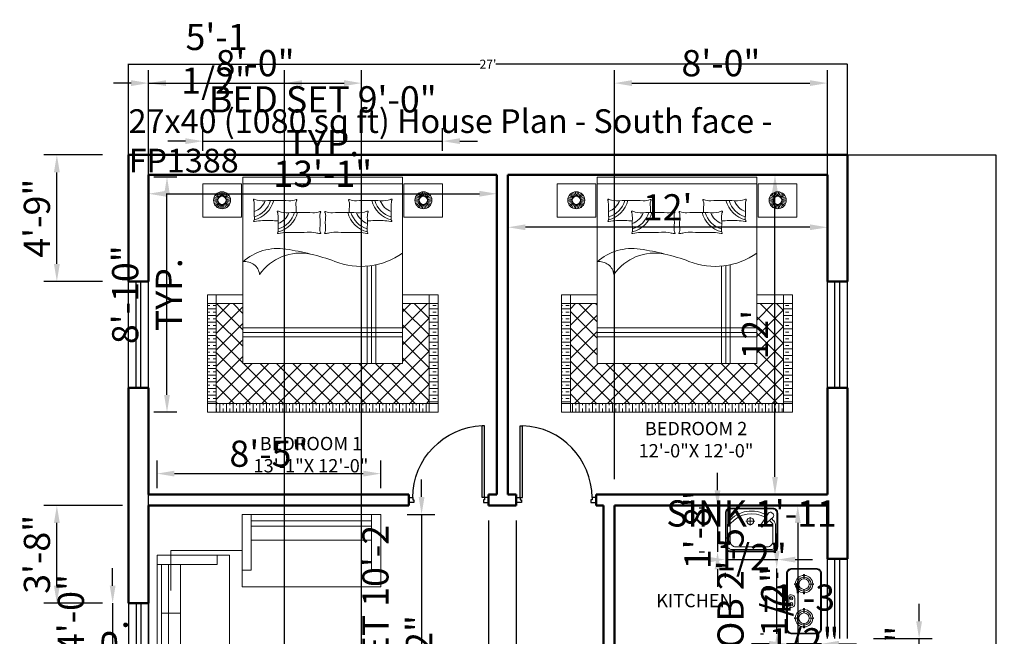
# Model space of a CAD drawing. Units: inches. Extents: x 117606 to 118050, y 251709 to 252357.
# Tile 3 of 3: x 117606 to 118050, y 252079 to 252357. Entities that reach past the tile are written whole.
import ezdxf

# ---------------------------------------------------------------- set-up
doc = ezdxf.new("R2010")
doc.units = ezdxf.units.IN
doc.header["$MEASUREMENT"] = 0
for name, color, linetype, lineweight in [('A-ANNO-TEXT', 7, 'Continuous', 25), ('A-AREA-IDEN', 7, 'Continuous', 25), ('A-DOOR', 4, 'Continuous', 25), ('A-EQPM', 9, 'Continuous', 18), ('FURNITURE', 53, 'Continuous', 18), ('SANITARY', 151, 'Continuous', 18), ('WALL', 7, 'Continuous', 50), ('WINDOW', 2, 'Continuous', 25), ('YQ_DIM', 3, 'Continuous', 18)]:
    doc.layers.add(name, color=color, linetype=linetype, lineweight=lineweight)
doc.styles.get("Standard").update_dxf_attribs({"font": 'arial.ttf'})
doc.styles.add('YQ_DIM', font='SUPEROS.SHX', dxfattribs={"width": 0.8, "bigfont": 'HZDX.SHX'})
doc.dimstyles.get("Standard").update_dxf_attribs({"dimtxt": 4, "dimasz": 0.18, "dimexe": 0.18, "dimexo": 0.0625, "dimgap": 0.09, "dimtad": 0, "dimtih": 1, "dimtoh": 1, "dimzin": 0, "dimdsep": 46, "dimlunit": 4, "dimtxsty": 'Standard', "dimcen": 0.09, "dimadec": 0, "dimazin": 0, "dimtfac": 1, "dimtofl": 0, "dimtmove": 0, "dimatfit": 3, "dimfxl": 1, "dimtolj": 1, "dimtzin": 0, "dimarcsym": 0})
doc.dimstyles.new('yqi3_937', dxfattribs={"dimscale": 3.937008, "dimtxt": 3, "dimasz": 2, "dimexe": 1.5, "dimexo": 3, "dimgap": 0.5, "dimtad": 1, "dimdsep": 46, "dimlunit": 4, "dimtxsty": 'YQ_DIM', "dimcen": 0, "dimclrd": 256, "dimclre": 256, "dimclrt": 7, "dimadec": 1, "dimazin": 2, "dimtfac": 1, "dimtix": 1, "dimtmove": 2, "dimatfit": 2, "dimfxl": 1, "dimtolj": 1, "dimtzin": 0, "dimarcsym": 0})

# ---------------------------------------------------------------- blocks, each defined once
blk = doc.blocks.new('*D1')
at = {"layer": 'Defpoints', "color": 0, "transparency": 16777216}
for p in [(117978.89, 252337.19), (117654.89, 252296.28), (117978.89, 252296.28)]:
    blk.add_point(p, dxfattribs=at)
at = {"layer": 'YQ_DIM', "color": 0, "lineweight": -2, "transparency": 16777216}
for p, q in [((117654.89, 252296.35), (117654.89, 252337.37)), ((117655.07, 252337.19), (117813.37, 252337.19)), ((117978.71, 252337.19), (117820.4, 252337.19)), ((117978.89, 252296.35), (117978.89, 252337.37))]:
    blk.add_line(p, q, dxfattribs=at)
at = {"layer": 'YQ_DIM', "color": 0, "transparency": 16777216}
for points in [[(117655.07, 252337.22), (117655.07, 252337.16), (117654.89, 252337.19)], [(117978.71, 252337.22), (117978.71, 252337.16), (117978.89, 252337.19)]]:
    blk.add_solid(points, dxfattribs=at)
at = {"layer": 'YQ_DIM', "color": 0, "transparency": 16777216, "insert": (117816.89, 252337.19), "char_height": 4, "attachment_point": 5}
blk.add_mtext("\\A1;27'", dxfattribs=at)
blk = doc.blocks.new('*D2')
at = {"layer": 'Defpoints', "color": 0, "transparency": 16777216}
for p in [(117978.89, 252296.28), (117978.89, 251816.28), (118045.85, 251816.28)]:
    blk.add_point(p, dxfattribs=at)
at = {"layer": 'YQ_DIM', "color": 0, "lineweight": -2, "transparency": 16777216}
for p, q in [((117978.95, 252296.28), (118046.03, 252296.28)), ((118045.85, 252296.1), (118045.85, 252058.42)), ((118045.85, 251816.46), (118045.85, 252054.15)), ((117978.95, 251816.28), (118046.03, 251816.28))]:
    blk.add_line(p, q, dxfattribs=at)
at = {"layer": 'YQ_DIM', "color": 0, "transparency": 16777216}
for points in [[(118045.82, 252296.1), (118045.88, 252296.1), (118045.85, 252296.28)], [(118045.82, 251816.46), (118045.88, 251816.46), (118045.85, 251816.28)]]:
    blk.add_solid(points, dxfattribs=at)
at = {"layer": 'YQ_DIM', "color": 0, "transparency": 16777216, "insert": (118045.85, 252056.28), "char_height": 4, "attachment_point": 5}
blk.add_mtext("\\A1;40'", dxfattribs=at)
blk = doc.blocks.new('*D4')
at = {"layer": 'Defpoints', "color": 0, "transparency": 16777216}
for p in [(117825.89, 252287.28), (117969.89, 252287.28), (117825.89, 252263.66)]:
    blk.add_point(p, dxfattribs=at)
at = {"layer": 'YQ_DIM', "color": 0, "lineweight": -2, "transparency": 16777216}
for p, q in [((117825.89, 252275.47), (117825.89, 252257.76)), ((117969.89, 252275.47), (117969.89, 252257.76)), ((117962.01, 252263.66), (117833.76, 252263.66))]:
    blk.add_line(p, q, dxfattribs=at)
at = {"layer": 'YQ_DIM', "color": 0, "transparency": 16777216}
for points in [[(117833.76, 252264.97), (117833.76, 252262.35), (117825.89, 252263.66)], [(117962.01, 252264.97), (117962.01, 252262.35), (117969.89, 252263.66)]]:
    blk.add_solid(points, dxfattribs=at)
at = {"layer": 'YQ_DIM', "color": 0, "transparency": 16777216, "insert": (117897.89, 252272.66), "char_height": 11.811, "attachment_point": 5, "style": 'YQ_DIM'}
blk.add_mtext("\\A1;12'", dxfattribs=at)
blk = doc.blocks.new('*D5')
at = {"layer": 'Defpoints', "color": 0, "transparency": 16777216}
for p in [(117946.26, 252287.28), (117969.89, 252287.28), (117969.89, 252143.28)]:
    blk.add_point(p, dxfattribs=at)
at = {"layer": 'YQ_DIM', "color": 0, "lineweight": -2, "transparency": 16777216}
for p, q in [((117958.07, 252287.28), (117940.36, 252287.28)), ((117946.26, 252151.16), (117946.26, 252279.41)), ((117958.07, 252143.28), (117940.36, 252143.28))]:
    blk.add_line(p, q, dxfattribs=at)
at = {"layer": 'YQ_DIM', "color": 0, "transparency": 16777216}
for points in [[(117944.95, 252279.41), (117947.58, 252279.41), (117946.26, 252287.28)], [(117944.95, 252151.16), (117947.58, 252151.16), (117946.26, 252143.28)]]:
    blk.add_solid(points, dxfattribs=at)
at = {"layer": 'YQ_DIM', "color": 0, "transparency": 16777216, "insert": (117937.26, 252215.28), "char_height": 11.811, "attachment_point": 5, "rotation": 90, "style": 'YQ_DIM'}
blk.add_mtext("\\A1;12'", dxfattribs=at)
blk = doc.blocks.new('*D9')
at = {"layer": 'Defpoints', "color": 0, "transparency": 16777216}
for p in [(117969.89, 252138.28), (117956.53, 252054.28), (117969.89, 252054.28)]:
    blk.add_point(p, dxfattribs=at)
at = {"layer": 'YQ_DIM', "color": 0, "lineweight": -2, "transparency": 16777216}
for p, q in [((117958.07, 252138.28), (117950.63, 252138.28)), ((117956.53, 252130.41), (117956.53, 252062.16)), ((117958.07, 252054.28), (117950.63, 252054.28))]:
    blk.add_line(p, q, dxfattribs=at)
at = {"layer": 'YQ_DIM', "color": 0, "transparency": 16777216}
for points in [[(117955.22, 252130.41), (117957.84, 252130.41), (117956.53, 252138.28)], [(117955.22, 252062.16), (117957.84, 252062.16), (117956.53, 252054.28)]]:
    blk.add_solid(points, dxfattribs=at)
at = {"layer": 'YQ_DIM', "color": 0, "transparency": 16777216, "insert": (117947.53, 252096.28), "char_height": 11.811, "attachment_point": 5, "rotation": 90, "style": 'YQ_DIM'}
blk.add_mtext("\\A1;7'", dxfattribs=at)
blk = doc.blocks.new('DR_D01')
for p, q in [((-0.45, 0.93), (-0.42, 0.93)), ((-0.45, 0.03), (-0.45, 0.93)), ((-0.42, 0.03), (-0.42, 0.93)), ((-0.5, 0.03), (-0.42, 0.03)), ((-0.5, 0.03), (-0.5, -0.03)), ((-0.45, 0.03), (-0.45, 0)), ((-0.45, 0), (-0.435, 0)), ((-0.435, 0), (-0.435, -0.03)), ((0.435, 0), (0.435, -0.03)), ((0.45, 0), (0.435, 0)), ((0.45, 0.03), (0.45, 0)), ((0.5, 0.03), (0.45, 0.03)), ((0.5, -0.03), (0.5, 0.03)), ((-0.435, -0.03), (-0.5, -0.03)), ((0.435, -0.03), (0.5, -0.03))]:
    blk.add_line(p, q)
blk.add_arc((-0.46, 0.021), 0.91, 0.5915, 87.4664)
blk = doc.blocks.new('WD_WIN4')
for p, q in [((-0.5, 0.5), (0.5, 0.5)), ((-0.5, 0.12), (0.5, 0.12)), ((-0.5, -0.12), (0.5, -0.12)), ((-0.5, -0.5), (0.5, -0.5))]:
    blk.add_line(p, q)
blk = doc.blocks.new('BED')
h = blk.add_hatch()
h.set_pattern_fill('TRANS', color=256, scale=12, style=0)
h.set_pattern_definition([(360, (4433.967, -9715.0492), (1e-15, 3), []), (360, (4433.967, -9713.5492), (1e-15, 3), [1.5, -1.5])])
h.paths.add_polyline_path([(48, -103), (52, -103), (52, -58), (48, -58)])
h.paths.add_polyline_path([(-48, -58), (-52, -58), (-52, -103), (-48, -103)])
h = blk.add_hatch()
h.set_pattern_fill('ANSI37', color=256, scale=42, angle=-90, style=0)
h.set_pattern_definition([(315, (7787.1367, 4477.8466), (3.7123106, 3.7123106), []), (45, (7787.1367, 4477.8466), (-3.7123106, 3.7123106), [])])
h.paths.add_polyline_path([(-36, -85), (-36, -58), (-48, -58), (-48, -103), (48, -103), (48, -58), (36, -58), (36, -85)])
h = blk.add_hatch()
h.set_pattern_fill('TRANS', color=256, scale=12, angle=-90, style=0)
h.set_pattern_definition([(270, (4433.967, -9715.0492), (3, -1e-15), []), (270, (4435.467, -9715.0492), (3, -1e-15), [1.5, -1.5])])
h.paths.add_polyline_path([(48, -107), (48, -103), (-48, -103), (-48, -107)])
for p, q in [((-54, -4), (-54, -19)), ((-36.64, -4), (-54, -4)), ((-36.64, -4), (-36.64, -19)), ((-36, -1), (36, -1)), ((-36, -85), (-36, -1)), ((-36, -4), (36, -4)), ((36, -1), (36, -85)), ((36.64, -4), (36.64, -19)), ((36.64, -4), (54, -4)), ((54, -4), (54, -19)), ((-46.62, -10.08), (-47.96, -8.6)), ((-46.31, -9.86), (-47.31, -8.13)), ((-45.96, -9.7), (-46.58, -7.8)), ((-45.58, -9.62), (-45.8, -7.63)), ((-45.2, -9.62), (-45, -7.63)), ((-44.82, -9.7), (-44.21, -7.79)), ((-44.47, -9.85), (-43.48, -8.12)), ((-44.16, -10.08), (-42.83, -8.59)), ((44.16, -10.08), (42.83, -8.59)), ((44.47, -9.85), (43.48, -8.12)), ((44.82, -9.7), (44.21, -7.79)), ((45.2, -9.62), (45, -7.63)), ((45.58, -9.62), (45.8, -7.63)), ((45.96, -9.7), (46.58, -7.8)), ((46.31, -9.86), (47.31, -8.13)), ((46.62, -10.08), (47.96, -8.6)), ((-47.23, -11.45), (-49.23, -11.45)), ((-47.19, -11.07), (-49.14, -10.66)), ((-47.19, -11.83), (-49.14, -12.25)), ((-47.07, -10.7), (-48.9, -9.89)), ((-47.07, -12.2), (-48.89, -13.01)), ((-46.88, -10.37), (-48.5, -9.2)), ((-46.87, -12.53), (-48.49, -13.71)), ((-46.62, -12.81), (-47.95, -14.3)), ((-46.3, -13.04), (-47.3, -14.77)), ((-45.95, -13.2), (-46.57, -15.1)), ((-45.58, -13.27), (-45.78, -15.26)), ((-45.19, -13.27), (-44.98, -15.26)), ((-44.82, -13.19), (-44.2, -15.09)), ((-44.47, -13.04), (-43.46, -14.77)), ((-44.16, -12.81), (-42.82, -14.29)), ((-43.9, -10.36), (-42.29, -9.18)), ((-43.9, -12.52), (-42.28, -13.7)), ((-43.71, -10.7), (-41.89, -9.88)), ((-43.71, -12.19), (-41.88, -13)), ((-43.59, -11.06), (-41.64, -10.64)), ((-43.59, -11.83), (-41.63, -12.24)), ((-43.55, -11.44), (-41.55, -11.44)), ((43.55, -11.44), (41.55, -11.44)), ((43.59, -11.83), (41.63, -12.24)), ((43.59, -11.06), (41.64, -10.64)), ((43.71, -12.19), (41.88, -13)), ((43.71, -10.7), (41.89, -9.88)), ((43.9, -12.52), (42.28, -13.7)), ((43.9, -10.36), (42.29, -9.18)), ((44.16, -12.81), (42.82, -14.29)), ((44.47, -13.04), (43.46, -14.77)), ((44.82, -13.19), (44.2, -15.09)), ((45.19, -13.27), (44.98, -15.26)), ((45.58, -13.27), (45.78, -15.26)), ((45.95, -13.2), (46.57, -15.1)), ((46.3, -13.04), (47.3, -14.77)), ((46.62, -12.81), (47.95, -14.3)), ((46.87, -12.53), (48.49, -13.71)), ((46.88, -10.37), (48.5, -9.2)), ((47.07, -10.7), (48.9, -9.89)), ((47.07, -12.2), (48.89, -13.01)), ((47.19, -11.07), (49.14, -10.66)), ((47.19, -11.83), (49.14, -12.25)), ((47.23, -11.45), (49.23, -11.45)), ((-36.64, -19), (-54, -19)), ((36.64, -19), (54, -19)), ((20, -85), (20, -41.14)), ((22, -85), (22, -40.91)), ((24, -85), (24, -40.55)), ((-52, -54), (-52, -107)), ((-52, -54), (-36, -54)), ((-48, -54), (-48, -107)), ((36, -54), (52, -54)), ((48, -54), (48, -107)), ((52, -54), (52, -107)), ((-52, -58), (-36, -58)), ((36, -58), (52, -58)), ((36, -69), (-36, -69)), ((36, -71), (-36, -71)), ((36, -73), (-36, -73)), ((36, -85), (-36, -85)), ((-52, -103), (52, -103)), ((-52, -107), (52, -107))]:
    blk.add_line(p, q)
for centre, radius in [((-45.39, -11.45), 3.84), ((45.39, -11.45), 3.84), ((-45.39, -11.45), 1.84), ((45.39, -11.45), 1.84)]:
    blk.add_circle(centre, radius)
for centre, radius, start, end in [((-30.92, -11.24), 0.328, 35.8976, 208.6272), ((-42.38, -17.5), 12.73, 27.1629, 28.6272), ((-44.37, -13.89), 13.5, 357.4804, 9.3956), ((-33.8, -8.61), 8.46, 289.8695, 338.9843), ((-33.8, -8.61), 12.06, 283.8498, 346.0842), ((-33.8, -8.61), 10.71, 286.0319, 344.1205), ((-26.84, 0.13), 11.82, 251.1782, 273.3982), ((-20.92, -99.64), 88.13, 86.2964, 93.3982), ((-14.79, -4.98), 6.73, 266.2964, 294.303), ((-8.24, -13.16), 3.86, 159.0146, 186.273), ((-11.92, -11.33), 0.242, 335.7259, 114.303), ((-5.69, -14.14), 6.59, 155.7259, 159.0146), ((11.92, -11.33), 0.242, 65.697, 204.2741), ((5.69, -14.14), 6.59, 20.9854, 24.2741), ((8.24, -13.16), 3.86, 353.727, 20.9854), ((14.79, -4.98), 6.73, 245.697, 273.7036), ((20.92, -99.64), 88.13, 86.6018, 93.7036), ((33.8, -8.61), 12.06, 193.9158, 256.1502), ((33.8, -8.61), 10.71, 195.8795, 253.9681), ((33.8, -8.61), 8.46, 201.0157, 250.1305), ((26.84, 0.13), 11.82, 266.6018, 288.8218), ((30.92, -11.24), 0.328, 331.3728, 144.1024), ((44.37, -13.89), 13.5, 170.6044, 182.5196), ((42.38, -17.5), 12.73, 151.3728, 152.8371), ((10.15, -16.29), 41.07, 177.4804, 184.5075), ((-20.16, -16.62), 0.328, 35.8976, 208.6272), ((-31.62, -22.87), 12.73, 27.1629, 28.6272), ((-33.61, -19.26), 13.5, 357.4804, 9.3956), ((-23.04, -13.99), 8.46, 289.8695, 338.9843), ((-23.04, -13.99), 12.06, 283.8498, 346.0842), ((-23.04, -13.99), 10.71, 286.0319, 344.1205), ((-16.08, -5.24), 11.82, 251.1782, 273.3982), ((-10.15, -105.01), 88.13, 86.2964, 93.3982), ((-36.64, -16.28), 24.71, 358.5721, 6.273), ((-4.03, -10.35), 6.73, 266.2964, 294.303), ((2.52, -18.53), 3.86, 159.0146, 186.273), ((-1.16, -16.7), 0.242, 335.7259, 114.303), ((5.07, -19.51), 6.59, 155.7259, 159.0146), ((1.16, -16.7), 0.242, 65.697, 204.2741), ((-5.07, -19.51), 6.59, 20.9854, 24.2741), ((-2.52, -18.53), 3.86, 353.727, 20.9854), ((4.03, -10.35), 6.73, 245.697, 273.7036), ((10.15, -105.01), 88.13, 86.6018, 93.7036), ((23.04, -13.99), 12.06, 193.9158, 256.1502), ((36.64, -16.28), 24.71, 173.727, 181.4279), ((23.04, -13.99), 10.71, 195.8795, 253.9681), ((23.04, -13.99), 8.46, 201.0157, 250.1305), ((16.08, -5.24), 11.82, 266.6018, 288.8218), ((20.16, -16.62), 0.328, 331.3728, 144.1024), ((33.61, -19.26), 13.5, 170.6044, 182.5196), ((31.62, -22.87), 12.73, 151.3728, 152.8371), ((-10.15, -16.29), 41.07, 355.4925, 2.5196), ((-30.88, -20.82), 0.25, 147.6219, 311.9343), ((-32.72, -19.65), 1.93, 327.6219, 339.2246), ((-32.67, -19.67), 1.88, 339.2246, 4.5075), ((-25.16, -53.53), 33, 93.5164, 99.6766), ((-25.27, -51.86), 31.33, 86.4836, 93.5164), ((-21.12, 15.68), 36.34, 266.4836, 271.5234), ((20.91, -21.66), 41.07, 177.4804, 184.5075), ((-25.88, -21.66), 24.71, 354.3784, 6.273), ((25.88, -21.66), 24.71, 173.727, 185.6216), ((-20.91, -21.66), 41.07, 355.4925, 2.5196), ((21.12, 15.68), 36.34, 268.4766, 273.5164), ((25.27, -51.86), 31.33, 86.4836, 93.5164), ((25.16, -53.53), 33, 80.3234, 86.4836), ((30.88, -20.82), 0.25, 228.0657, 32.3781), ((32.67, -19.67), 1.88, 175.4925, 200.7754), ((32.72, -19.65), 1.93, 200.7754, 212.3781), ((-20.12, -26.19), 0.25, 147.6219, 311.9343), ((-21.96, -25.02), 1.93, 327.6219, 339.2246), ((-21.91, -25.04), 1.88, 339.2246, 4.5075), ((-14.4, -58.9), 33, 93.5164, 99.6766), ((-14.51, -57.23), 31.33, 86.4836, 93.5164), ((-10.35, 10.3), 36.34, 266.4836, 275.306), ((-5.78, -38.98), 13.15, 77.9645, 95.306), ((2.5, -0.17), 26.53, 257.9645, 261.9243), ((2.55, -24.46), 3.86, 174.3784, 204.7617), ((-1.09, -26.25), 0.228, 231.9005, 52.8902), ((1.09, -26.25), 0.228, 127.1098, 308.0995), ((-2.55, -24.46), 3.86, 335.2383, 5.6216), ((-2.5, -0.17), 26.53, 278.0757, 282.0355), ((5.78, -38.98), 13.15, 84.694, 102.0355), ((10.35, 10.3), 36.34, 264.694, 273.5164), ((14.51, -57.23), 31.33, 86.4836, 93.5164), ((14.4, -58.9), 33, 80.3234, 86.4836), ((20.12, -26.19), 0.25, 228.0657, 32.3781), ((21.91, -25.04), 1.88, 175.4925, 200.7754), ((21.96, -25.02), 1.93, 200.7754, 212.3781), ((-20.27, -56.85), 23.66, 81.0857, 131.6581), ((-9.91, -57.83), 22.61, 78.6456, 145.1521), ((-32.56, -143.87), 111.55, 70.0977, 81.7735), ((17.27, -9.21), 32.05, 248.2778, 305.7663), ((-34.97, -45.63), 6.55, 6.3172, 99.0807)]:
    blk.add_arc(centre, radius, start, end)
blk = doc.blocks.new('*D25')
at = {"layer": 'Defpoints', "color": 0, "transparency": 16777216}
for p in [(117663.89, 252287.28), (117820.89, 252287.28), (117820.89, 252278.78)]:
    blk.add_point(p, dxfattribs=at)
at = {"layer": 'YQ_DIM', "color": 0, "lineweight": -2, "transparency": 16777216}
for p, q in [((117671.76, 252278.78), (117813.01, 252278.78)), ((117663.89, 252275.47), (117663.89, 252272.88)), ((117820.89, 252275.47), (117820.89, 252272.88))]:
    blk.add_line(p, q, dxfattribs=at)
at = {"layer": 'YQ_DIM', "color": 0, "transparency": 16777216}
for points in [[(117671.76, 252280.09), (117671.76, 252277.47), (117663.89, 252278.78)], [(117813.01, 252280.09), (117813.01, 252277.47), (117820.89, 252278.78)]]:
    blk.add_solid(points, dxfattribs=at)
at = {"layer": 'YQ_DIM', "color": 0, "transparency": 16777216, "insert": (117742.39, 252287.78), "char_height": 11.811, "attachment_point": 5, "style": 'YQ_DIM'}
blk.add_mtext('\\A1;13\'-1"', dxfattribs=at)
blk = doc.blocks.new('yq_cooker_01')
for p, q in [((426, 34), (466, 34)), ((426, -34), (466, -34))]:
    blk.add_line(p, q)
for points in [[(440, -375), (160, -375, -0.414214), (100, -315), (100, 315, -0.414214), (160, 375), (440, 375, -0.414214), (500, 315), (500, -315, -0.414214)], [(440, -365), (160, -365, -0.414214), (110, -315), (110, 315, -0.414214), (160, 365), (440, 365, -0.414214), (490, 315), (490, -315, -0.414214)]]:
    blk.add_lwpolyline(points, format="xyb", close=True)
for points in [[(301, 261), (305, 305), (295, 305), (299, 261)], [(234, 196), (190, 200), (190, 190), (234, 194)], [(299, 129), (295, 85), (305, 85), (301, 129)], [(366, 194), (410, 190), (410, 200), (366, 196)], [(299, -129), (295, -85), (305, -85), (301, -129)], [(234, -196), (190, -200), (190, -190), (234, -194)], [(366, -194), (410, -190), (410, -200), (366, -196)], [(301, -261), (305, -305), (295, -305), (299, -261)]]:
    blk.add_lwpolyline(points, close=True)
blk.add_lwpolyline([(407, -34, 0.414214), (446, -73), (456, -73, 0.414214), (475, -54), (475, 54, 0.414214), (456, 74), (446, 74, 0.414214), (407, 34), (407, -34)], format="xyb")
for centre, radius in [((300, 195), 60), ((446, 34), 19.6), ((446, -34), 19.6), ((300, -195), 60)]:
    blk.add_circle(centre, radius)
for centre, radius, start, end in [((300, 195), 100, 92.4978, 177.5022), ((300, 195), 80, 91.5913, 178.4087), ((300, 195), 80, 1.5913, 88.4087), ((300, 195), 100, 2.4978, 87.5022), ((300, 195), 100, 182.4978, 267.5022), ((300, 195), 80, 181.5913, 268.4087), ((300, 195), 80, 271.5913, 358.4087), ((300, 195), 100, 272.4978, 357.5022), ((300, -195), 100, 92.4978, 177.5022), ((300, -195), 100, 2.4978, 87.5022), ((300, -195), 100, 182.4978, 267.5022), ((300, -195), 80, 91.5913, 178.4087), ((300, -195), 80, 181.5913, 268.4087), ((300, -195), 80, 1.5913, 88.4087), ((300, -195), 80, 271.5913, 358.4087), ((300, -195), 100, 272.4978, 357.5022)]:
    blk.add_arc(centre, radius, start, end)
blk = doc.blocks.new('yq_ksink_01')
for points in [[(540, -243), (540, 243, 0.414214), (483, 300), (97, 300, 0.414214), (40, 243), (40, -243, 0.414214), (97, -300), (483, -300, 0.414214)], [(530, -243), (530, 243, 0.414214), (483, 290), (97, 290, 0.414214), (50, 243), (50, -243, 0.414214), (97, -290), (483, -290, 0.414214)], [(142, 246, 0.463705), (106, 246), (93, 231, 0.463199), (99, 196), (244, 99), (260, 117)]]:
    blk.add_lwpolyline(points, format="xyb", close=True)
for points in [[(124, 179, 0.371537), (197, -263, 0.175756), (227, -274), (468, -274, 0.414214), (514, -228), (514, 228, 0.414214), (468, 274), (227, 274, 0.175756), (197, 263, 0.038636), (159, 226, 0.038636)], [(149, 162, 0.370424), (217, -240, 0.175756), (227, -244), (421, -244, 0.414214), (484, -181), (484, 181, 0.414214), (421, 244), (227, 244, 0.175756), (217, 240, 0.038502), (180, 204, 0.038502)]]:
    blk.add_lwpolyline(points, format="xyb")
for points in [[(191, -64), (191, 36)], [(142, -14), (241, -14)]]:
    blk.add_lwpolyline(points)
blk.add_circle((191, -14), 38.3)
blk = doc.blocks.new('A$C4d06a8b4')
for p, q in [((27.06, 122.57), (27.06, 118.4)), ((27.06, 118.4), (0, 118.4)), ((2.07, 96.36), (2.07, 118.4)), ((5.25, 118.4), (5.25, 22.51)), ((10.59, 118.4), (10.59, 22.51)), ((10.59, 96.36), (2.07, 96.36)), ((2.07, 96.36), (2.07, 70.46)), ((2.07, 70.46), (10.59, 70.46)), ((2.07, 44.55), (2.07, 70.46)), ((10.59, 70.46), (32.66, 70.46)), ((10.59, 44.55), (2.07, 44.55)), ((2.07, 44.55), (2.07, 22.51)), ((27.06, 22.51), (0, 22.51)), ((27.06, 18.34), (27.06, 22.51)), ((42.51, 25.08), (38.34, 25.08)), ((42.51, 25.08), (42.51, 0)), ((96.71, 25.08), (96.71, 0)), ((96.71, 25.08), (100.88, 25.08)), ((42.51, 11.63), (96.71, 11.63)), ((96.71, 5.25), (42.51, 5.25)), ((42.51, 2.89), (96.71, 2.89))]:
    blk.add_line(p, q)
for points in [[(32.66, 122.57), (32.66, 18.34), (0, 18.34), (0, 122.57)], [(38.34, 0), (100.88, 0), (100.88, 32.66), (38.34, 32.66)]]:
    blk.add_lwpolyline(points, close=True)
at = {"color": 0, "linetype": 'ByBlock', "lineweight": -2}
blk.add_lwpolyline([(86.22, 60.81), (86.22, 111.84), (60.71, 111.84), (60.71, 60.81)], close=True, dxfattribs=at)
for points in [[(6.25, 16.33), (6.25, 34.21)], [(38.34, 16.33), (6.25, 16.33)]]:
    blk.add_lwpolyline(points, dxfattribs=at)
blk = doc.blocks.new('*D141')
at = {"layer": 'Defpoints', "color": 0, "transparency": 16777216}
for p in [(117654.89, 252094.28), (117647.69, 252046.28), (117654.89, 252046.28)]:
    blk.add_point(p, dxfattribs=at)
at = {"layer": 'YQ_DIM', "lineweight": -2, "transparency": 16777216}
for p, q in [((117647.69, 252102.16), (117647.69, 252110.03)), ((117643.07, 252094.28), (117641.78, 252094.28)), ((117647.69, 252094.28), (117647.69, 252046.28)), ((117643.07, 252046.28), (117641.78, 252046.28)), ((117647.69, 252038.41), (117647.69, 252030.54))]:
    blk.add_line(p, q, dxfattribs=at)
at = {"layer": 'YQ_DIM', "transparency": 16777216}
for points in [[(117646.37, 252102.16), (117649, 252102.16), (117647.69, 252094.28)], [(117646.37, 252038.41), (117649, 252038.41), (117647.69, 252046.28)]]:
    blk.add_solid(points, dxfattribs=at)
at = {"layer": 'YQ_DIM', "color": 7, "transparency": 16777216, "insert": (117638.69, 252070.28), "char_height": 11.811, "attachment_point": 5, "rotation": 90, "style": 'YQ_DIM'}
blk.add_mtext('\\A1;WIN. 4\'-0" TYP.', dxfattribs=at)
blk = doc.blocks.new('*D151')
at = {"layer": 'Defpoints', "color": 0, "transparency": 16777216}
for p in [(117796.39, 252302.48), (117688.39, 252286.28), (117796.39, 252286.28)]:
    blk.add_point(p, dxfattribs=at)
at = {"layer": 'YQ_DIM', "lineweight": -2, "transparency": 16777216}
for p, q in [((117688.39, 252298.1), (117688.39, 252308.39)), ((117796.39, 252298.1), (117796.39, 252308.39)), ((117680.51, 252302.48), (117672.64, 252302.48)), ((117688.39, 252302.48), (117796.39, 252302.48)), ((117804.26, 252302.48), (117812.13, 252302.48))]:
    blk.add_line(p, q, dxfattribs=at)
at = {"layer": 'YQ_DIM', "transparency": 16777216}
for points in [[(117680.51, 252303.8), (117680.51, 252301.17), (117688.39, 252302.48)], [(117804.26, 252303.8), (117804.26, 252301.17), (117796.39, 252302.48)]]:
    blk.add_solid(points, dxfattribs=at)
at = {"layer": 'YQ_DIM', "color": 7, "transparency": 16777216, "insert": (117742.39, 252311.48), "char_height": 11.811, "attachment_point": 5, "style": 'YQ_DIM'}
blk.add_mtext('\\A1;BED SET 9\'-0" TYP.', dxfattribs=at)
blk = doc.blocks.new('*D152')
at = {"layer": 'Defpoints', "color": 0, "transparency": 16777216}
for p in [(117672.19, 252286.28), (117688.39, 252286.28), (117688.39, 252180.28)]:
    blk.add_point(p, dxfattribs=at)
at = {"layer": 'YQ_DIM', "lineweight": -2, "transparency": 16777216}
for p, q in [((117676.57, 252286.28), (117666.28, 252286.28)), ((117672.19, 252188.16), (117672.19, 252278.41)), ((117676.57, 252180.28), (117666.28, 252180.28))]:
    blk.add_line(p, q, dxfattribs=at)
at = {"layer": 'YQ_DIM', "transparency": 16777216}
for points in [[(117670.87, 252278.41), (117673.5, 252278.41), (117672.19, 252286.28)], [(117670.87, 252188.16), (117673.5, 252188.16), (117672.19, 252180.28)]]:
    blk.add_solid(points, dxfattribs=at)
at = {"layer": 'YQ_DIM', "color": 7, "transparency": 16777216, "insert": (117663.19, 252233.28), "char_height": 11.811, "attachment_point": 5, "rotation": 90, "style": 'YQ_DIM'}
blk.add_mtext('\\A1;8\'-10" TYP.', dxfattribs=at)
blk = doc.blocks.new('*D153')
at = {"layer": 'Defpoints', "color": 0, "transparency": 16777216}
for p in [(117947.05, 252109.93), (117951.48, 252109.93), (117951.48, 252080.4)]:
    blk.add_point(p, dxfattribs=at)
at = {"layer": 'YQ_DIM', "lineweight": -2, "transparency": 16777216}
for p, q in [((117947.05, 252117.8), (117947.05, 252125.68)), ((117939.67, 252109.93), (117941.15, 252109.93)), ((117947.05, 252080.4), (117947.05, 252109.93)), ((117939.67, 252080.4), (117941.15, 252080.4)), ((117947.05, 252072.53), (117947.05, 252064.66))]:
    blk.add_line(p, q, dxfattribs=at)
at = {"layer": 'YQ_DIM', "transparency": 16777216}
for points in [[(117945.74, 252117.8), (117948.36, 252117.8), (117947.05, 252109.93)], [(117945.74, 252072.53), (117948.36, 252072.53), (117947.05, 252080.4)]]:
    blk.add_solid(points, dxfattribs=at)
at = {"layer": 'YQ_DIM', "color": 7, "transparency": 16777216, "insert": (117936.08, 252095.17), "char_height": 11.811, "attachment_point": 5, "rotation": 90, "style": 'YQ_DIM'}
blk.add_mtext('\\A1;HOB 2\'-5 1/2"', dxfattribs=at)
blk = doc.blocks.new('*D154')
at = {"layer": 'Defpoints', "color": 0, "transparency": 16777216}
for p in [(117951.48, 252080.4), (117967.23, 252080.4), (117951.48, 252075.97)]:
    blk.add_point(p, dxfattribs=at)
at = {"layer": 'YQ_DIM', "lineweight": -2, "transparency": 16777216}
for p, q in [((117943.61, 252075.97), (117935.73, 252075.97)), ((117967.23, 252075.97), (117951.48, 252075.97)), ((117975.1, 252075.97), (117982.98, 252075.97)), ((117951.48, 252068.59), (117951.48, 252070.07)), ((117967.23, 252068.59), (117967.23, 252070.07))]:
    blk.add_line(p, q, dxfattribs=at)
at = {"layer": 'YQ_DIM', "transparency": 16777216}
for points in [[(117943.61, 252077.29), (117943.61, 252074.66), (117951.48, 252075.97)], [(117975.1, 252077.29), (117975.1, 252074.66), (117967.23, 252075.97)]]:
    blk.add_solid(points, dxfattribs=at)
at = {"layer": 'YQ_DIM', "color": 7, "transparency": 16777216, "insert": (117959.36, 252086.94), "char_height": 11.811, "attachment_point": 5, "style": 'YQ_DIM'}
blk.add_mtext('\\A1;1\'-3 1/2"', dxfattribs=at)
blk = doc.blocks.new('*D155')
at = {"layer": 'Defpoints', "color": 0, "transparency": 16777216}
for p in [(117923.9, 252117.44), (117947.49, 252117.44), (117947.49, 252113.9)]:
    blk.add_point(p, dxfattribs=at)
at = {"layer": 'YQ_DIM', "lineweight": -2, "transparency": 16777216}
for p, q in [((117916.02, 252113.9), (117908.15, 252113.9)), ((117923.9, 252113.9), (117947.49, 252113.9)), ((117955.36, 252113.9), (117963.24, 252113.9)), ((117923.9, 252105.62), (117923.9, 252107.99)), ((117947.49, 252105.62), (117947.49, 252107.99))]:
    blk.add_line(p, q, dxfattribs=at)
at = {"layer": 'YQ_DIM', "transparency": 16777216}
for points in [[(117916.02, 252115.21), (117916.02, 252112.58), (117923.9, 252113.9)], [(117955.36, 252115.21), (117955.36, 252112.58), (117947.49, 252113.9)]]:
    blk.add_solid(points, dxfattribs=at)
at = {"layer": 'YQ_DIM', "color": 7, "transparency": 16777216, "insert": (117935.69, 252124.86), "char_height": 11.811, "attachment_point": 5, "style": 'YQ_DIM'}
blk.add_mtext('\\A1;SINK 1\'-11 1/2"', dxfattribs=at)
blk = doc.blocks.new('*D156')
at = {"layer": 'Defpoints', "color": 0, "transparency": 16777216}
for p in [(117923.9, 252137.28), (117920.36, 252117.44), (117923.9, 252117.44)]:
    blk.add_point(p, dxfattribs=at)
at = {"layer": 'YQ_DIM', "lineweight": -2, "transparency": 16777216}
for p, q in [((117920.36, 252145.16), (117920.36, 252153.03)), ((117912.09, 252137.28), (117914.45, 252137.28)), ((117920.36, 252137.28), (117920.36, 252117.44)), ((117912.09, 252117.44), (117914.45, 252117.44)), ((117920.36, 252109.56), (117920.36, 252101.69))]:
    blk.add_line(p, q, dxfattribs=at)
at = {"layer": 'YQ_DIM', "transparency": 16777216}
for points in [[(117919.04, 252145.16), (117921.67, 252145.16), (117920.36, 252137.28)], [(117919.04, 252109.56), (117921.67, 252109.56), (117920.36, 252117.44)]]:
    blk.add_solid(points, dxfattribs=at)
at = {"layer": 'YQ_DIM', "color": 7, "transparency": 16777216, "insert": (117911.36, 252127.36), "char_height": 11.811, "attachment_point": 5, "rotation": 90, "style": 'YQ_DIM'}
blk.add_mtext('\\A1;1\'-8"', dxfattribs=at)
blk = doc.blocks.new('*D159')
at = {"layer": 'Defpoints', "color": 0, "transparency": 16777216}
for p in [(117768.57, 252134.27), (117768.57, 252011.7), (117786.95, 252011.7)]:
    blk.add_point(p, dxfattribs=at)
at = {"layer": 'YQ_DIM', "lineweight": -2, "transparency": 16777216}
for p, q in [((117786.95, 252142.14), (117786.95, 252150.02)), ((117780.38, 252134.27), (117792.86, 252134.27)), ((117786.95, 252134.27), (117786.95, 252011.7)), ((117780.38, 252011.7), (117792.86, 252011.7)), ((117786.95, 252003.82), (117786.95, 251995.95))]:
    blk.add_line(p, q, dxfattribs=at)
at = {"layer": 'YQ_DIM', "transparency": 16777216}
for points in [[(117785.64, 252142.14), (117788.26, 252142.14), (117786.95, 252134.27)], [(117785.64, 252003.82), (117788.26, 252003.82), (117786.95, 252011.7)]]:
    blk.add_solid(points, dxfattribs=at)
at = {"layer": 'YQ_DIM', "color": 7, "transparency": 16777216, "insert": (117775.98, 252072.98), "char_height": 11.811, "attachment_point": 5, "rotation": 90, "style": 'YQ_DIM'}
blk.add_mtext('\\A1;SOFA SET 10\'-2 1/2"', dxfattribs=at)
blk = doc.blocks.new('*D160')
at = {"layer": 'Defpoints', "color": 0, "transparency": 16777216}
for p in [(117768.57, 252152.65), (117667.69, 252134.27), (117768.57, 252134.27)]:
    blk.add_point(p, dxfattribs=at)
at = {"layer": 'YQ_DIM', "lineweight": -2, "transparency": 16777216}
for p, q in [((117667.69, 252146.08), (117667.69, 252158.56)), ((117768.57, 252146.08), (117768.57, 252158.56)), ((117675.56, 252152.65), (117760.69, 252152.65))]:
    blk.add_line(p, q, dxfattribs=at)
at = {"layer": 'YQ_DIM', "transparency": 16777216}
for points in [[(117675.56, 252153.97), (117675.56, 252151.34), (117667.69, 252152.65)], [(117760.69, 252153.97), (117760.69, 252151.34), (117768.57, 252152.65)]]:
    blk.add_solid(points, dxfattribs=at)
at = {"layer": 'YQ_DIM', "color": 7, "transparency": 16777216, "insert": (117718.13, 252161.65), "char_height": 11.811, "attachment_point": 5, "style": 'YQ_DIM'}
blk.add_mtext('\\A1;8\'-5"', dxfattribs=at)
blk = doc.blocks.new('*D165')
at = {"layer": 'Defpoints', "color": 0, "transparency": 16777216}
for p in [(117969.89, 252328.63), (117873.89, 252138.28), (117969.89, 252138.28)]:
    blk.add_point(p, dxfattribs=at)
at = {"layer": 'YQ_DIM', "lineweight": -2, "transparency": 16777216}
for p, q in [((117873.89, 252150.1), (117873.89, 252334.54)), ((117969.89, 252150.1), (117969.89, 252334.54)), ((117881.76, 252328.63), (117962.01, 252328.63))]:
    blk.add_line(p, q, dxfattribs=at)
at = {"layer": 'YQ_DIM', "transparency": 16777216}
for points in [[(117881.76, 252329.95), (117881.76, 252327.32), (117873.89, 252328.63)], [(117962.01, 252329.95), (117962.01, 252327.32), (117969.89, 252328.63)]]:
    blk.add_solid(points, dxfattribs=at)
at = {"layer": 'YQ_DIM', "color": 7, "transparency": 16777216, "insert": (117921.89, 252337.63), "char_height": 11.811, "attachment_point": 5, "style": 'YQ_DIM'}
blk.add_mtext('\\A1;8\'-0"', dxfattribs=at)
blk = doc.blocks.new('*D167')
at = {"layer": 'Defpoints', "color": 0, "transparency": 16777216}
for p in [(117622.54, 252138.28), (117663.89, 252138.28), (117654.89, 252094.28)]:
    blk.add_point(p, dxfattribs=at)
at = {"layer": 'YQ_DIM', "lineweight": -2, "transparency": 16777216}
for p, q in [((117652.07, 252138.28), (117616.63, 252138.28)), ((117622.54, 252102.16), (117622.54, 252130.41)), ((117643.07, 252094.28), (117616.63, 252094.28))]:
    blk.add_line(p, q, dxfattribs=at)
at = {"layer": 'YQ_DIM', "transparency": 16777216}
for points in [[(117621.22, 252130.41), (117623.85, 252130.41), (117622.54, 252138.28)], [(117621.22, 252102.16), (117623.85, 252102.16), (117622.54, 252094.28)]]:
    blk.add_solid(points, dxfattribs=at)
at = {"layer": 'YQ_DIM', "color": 7, "transparency": 16777216, "insert": (117613.54, 252116.28), "char_height": 11.811, "attachment_point": 5, "rotation": 90, "style": 'YQ_DIM'}
blk.add_mtext('\\A1;3\'-8"', dxfattribs=at)
blk = doc.blocks.new('*D168')
at = {"layer": 'Defpoints', "color": 0, "transparency": 16777216}
for p in [(117759.89, 252328.63), (117663.89, 251861.28), (117759.89, 251861.28)]:
    blk.add_point(p, dxfattribs=at)
at = {"layer": 'YQ_DIM', "lineweight": -2, "transparency": 16777216}
for p, q in [((117663.89, 251873.1), (117663.89, 252334.54)), ((117759.89, 251873.1), (117759.89, 252334.54)), ((117671.76, 252328.63), (117752.01, 252328.63))]:
    blk.add_line(p, q, dxfattribs=at)
at = {"layer": 'YQ_DIM', "transparency": 16777216}
for points in [[(117671.76, 252329.95), (117671.76, 252327.32), (117663.89, 252328.63)], [(117752.01, 252329.95), (117752.01, 252327.32), (117759.89, 252328.63)]]:
    blk.add_solid(points, dxfattribs=at)
at = {"layer": 'YQ_DIM', "color": 7, "transparency": 16777216, "insert": (117711.89, 252337.63), "char_height": 11.811, "attachment_point": 5, "style": 'YQ_DIM'}
blk.add_mtext('\\A1;8\'-0"', dxfattribs=at)
blk = doc.blocks.new('*D173')
at = {"layer": 'Defpoints', "color": 0, "transparency": 16777216}
for p in [(117622.54, 252296.28), (117654.89, 252296.28), (117654.89, 252239.28)]:
    blk.add_point(p, dxfattribs=at)
at = {"layer": 'YQ_DIM', "lineweight": -2, "transparency": 16777216}
for p, q in [((117643.07, 252296.28), (117616.63, 252296.28)), ((117622.54, 252247.16), (117622.54, 252288.41)), ((117643.07, 252239.28), (117616.63, 252239.28))]:
    blk.add_line(p, q, dxfattribs=at)
at = {"layer": 'YQ_DIM', "transparency": 16777216}
for points in [[(117621.22, 252288.41), (117623.85, 252288.41), (117622.54, 252296.28)], [(117621.22, 252247.16), (117623.85, 252247.16), (117622.54, 252239.28)]]:
    blk.add_solid(points, dxfattribs=at)
at = {"layer": 'YQ_DIM', "color": 7, "transparency": 16777216, "insert": (117613.54, 252267.78), "char_height": 11.811, "attachment_point": 5, "rotation": 90, "style": 'YQ_DIM'}
blk.add_mtext('\\A1;4\'-9"', dxfattribs=at)
blk = doc.blocks.new('*D179')
at = {"layer": 'Defpoints', "color": 0, "transparency": 16777216}
for p in [(117978.89, 252078.28), (118011.24, 252078.28), (117969.89, 252054.28)]:
    blk.add_point(p, dxfattribs=at)
at = {"layer": 'YQ_DIM', "lineweight": -2, "transparency": 16777216}
for p, q in [((118011.24, 252086.16), (118011.24, 252094.03)), ((117990.7, 252078.28), (118017.14, 252078.28)), ((118011.24, 252054.28), (118011.24, 252078.28)), ((117981.7, 252054.28), (118017.14, 252054.28)), ((118011.24, 252046.41), (118011.24, 252038.54))]:
    blk.add_line(p, q, dxfattribs=at)
at = {"layer": 'YQ_DIM', "transparency": 16777216}
for points in [[(118009.92, 252086.16), (118012.55, 252086.16), (118011.24, 252078.28)], [(118009.92, 252046.41), (118012.55, 252046.41), (118011.24, 252054.28)]]:
    blk.add_solid(points, dxfattribs=at)
at = {"layer": 'YQ_DIM', "color": 7, "transparency": 16777216, "insert": (118002.24, 252066.28), "char_height": 11.811, "attachment_point": 5, "rotation": 90, "style": 'YQ_DIM'}
blk.add_mtext('\\A1;2\'-0"', dxfattribs=at)
blk = doc.blocks.new('*D180')
at = {"layer": 'Defpoints', "color": 0, "transparency": 16777216}
for p in [(117725.19, 252328.63), (117663.89, 251997.28), (117725.19, 251997.28)]:
    blk.add_point(p, dxfattribs=at)
at = {"layer": 'YQ_DIM', "lineweight": -2, "transparency": 16777216}
for p, q in [((117663.89, 252009.1), (117663.89, 252334.54)), ((117725.19, 252009.1), (117725.19, 252334.54)), ((117656.01, 252328.63), (117648.14, 252328.63)), ((117663.89, 252328.63), (117725.19, 252328.63)), ((117733.06, 252328.63), (117740.94, 252328.63))]:
    blk.add_line(p, q, dxfattribs=at)
at = {"layer": 'YQ_DIM', "transparency": 16777216}
for points in [[(117656.01, 252329.95), (117656.01, 252327.32), (117663.89, 252328.63)], [(117733.06, 252329.95), (117733.06, 252327.32), (117725.19, 252328.63)]]:
    blk.add_solid(points, dxfattribs=at)
at = {"layer": 'YQ_DIM', "color": 7, "transparency": 16777216, "insert": (117694.54, 252339.6), "char_height": 11.811, "attachment_point": 5, "style": 'YQ_DIM'}
blk.add_mtext('\\A1;5\'-1 1/2"', dxfattribs=at)
blk = doc.blocks.new('*D182')
at = {"layer": 'Defpoints', "color": 0, "transparency": 16777216}
for p in [(117817.14, 252143.28), (117829.63, 252143.28), (117829.63, 251783.93)]:
    blk.add_point(p, dxfattribs=at)
at = {"layer": 'YQ_DIM', "lineweight": -2, "transparency": 16777216}
for p, q in [((117817.14, 252131.47), (117817.14, 251778.03)), ((117829.63, 252131.47), (117829.63, 251778.03)), ((117809.26, 251783.93), (117801.39, 251783.93)), ((117817.14, 251783.93), (117829.63, 251783.93)), ((117837.51, 251783.93), (117845.38, 251783.93))]:
    blk.add_line(p, q, dxfattribs=at)
at = {"layer": 'YQ_DIM', "transparency": 16777216}
for points in [[(117809.26, 251785.25), (117809.26, 251782.62), (117817.14, 251783.93)], [(117837.51, 251785.25), (117837.51, 251782.62), (117829.63, 251783.93)]]:
    blk.add_solid(points, dxfattribs=at)
at = {"layer": 'YQ_DIM', "color": 7, "transparency": 16777216, "insert": (117823.39, 251794.9), "char_height": 11.811, "attachment_point": 5, "style": 'YQ_DIM'}
blk.add_mtext('\\A1;1\'-0 1/2"', dxfattribs=at)

msp = doc.modelspace()

# ---------------------------------------------------------------- linework, layer by layer
at = {"layer": 'WALL'}
for p, q in [((117654.885, 252296.284), (117978.885, 252296.284)), ((117654.885, 252239.284), (117654.885, 252296.284)), ((117978.885, 252239.284), (117978.885, 252296.284)), ((117663.885, 252287.284), (117820.885, 252287.284)), ((117663.885, 252239.284), (117663.885, 252287.284)), ((117820.885, 252143.284), (117820.885, 252287.284)), ((117825.885, 252143.284), (117825.885, 252287.284)), ((117825.885, 252287.284), (117969.885, 252287.284)), ((117969.885, 252239.284), (117969.885, 252287.284)), ((117663.885, 252239.284), (117654.885, 252239.284)), ((117969.885, 252239.284), (117978.885, 252239.284)), ((117663.885, 252191.284), (117654.885, 252191.284)), ((117654.885, 252094.284), (117654.885, 252191.284)), ((117663.885, 252143.284), (117663.885, 252191.284)), ((117969.885, 252143.284), (117969.885, 252191.284)), ((117969.885, 252191.284), (117978.885, 252191.284)), ((117978.885, 252114.284), (117978.885, 252191.284)), ((117663.885, 252143.284), (117781.137, 252143.284)), ((117781.137, 252138.284), (117781.137, 252143.284)), ((117817.137, 252143.284), (117820.885, 252143.284)), ((117817.137, 252138.284), (117817.137, 252143.284)), ((117825.885, 252143.284), (117829.633, 252143.284)), ((117829.633, 252138.284), (117829.633, 252143.279)), ((117865.633, 252143.284), (117969.885, 252143.284)), ((117865.633, 252138.284), (117865.633, 252143.284)), ((117663.885, 252138.284), (117781.137, 252138.284)), ((117663.885, 252094.284), (117663.885, 252138.284)), ((117817.137, 252138.284), (117829.633, 252138.284)), ((117865.633, 252138.284), (117868.885, 252138.284)), ((117868.885, 252049.284), (117868.885, 252138.284)), ((117873.885, 252138.284), (117969.885, 252138.284)), ((117873.885, 252054.284), (117873.885, 252138.284)), ((117969.885, 252114.284), (117969.885, 252138.284)), ((117969.885, 252114.284), (117978.885, 252114.284)), ((117663.885, 252094.284), (117654.885, 252094.284))]:
    msp.add_line(p, q, dxfattribs=at)

# ---------------------------------------------------------------- block references
at = {"layer": 'A-DOOR', "yscale": -36, "zscale": 36, "rotation": 180}
for p, xscale in [((117799.137, 252140.784), 36), ((117847.633, 252140.779), -36)]:
    msp.add_blockref('DR_D01', p, dxfattribs=dict(at, xscale=xscale))
at = {"layer": 'A-EQPM', "xscale": 0.0393700787401575, "yscale": -0.0393700787401575, "zscale": 0.0393700787401575, "rotation": 179.999999999994}
msp.add_blockref('yq_cooker_01', (117971.166, 252095.167), dxfattribs=at)
at = {"layer": 'FURNITURE'}
for p in [(117742.385, 252287.284), (117902.084, 252287.284)]:
    msp.add_blockref('BED', p, dxfattribs=at)
at = {"layer": 'FURNITURE', "xscale": -1, "rotation": 180}
msp.add_blockref('A$C4d06a8b4', (117667.688, 252134.269), dxfattribs=at)
at = {"layer": 'SANITARY', "xscale": 0.0393700787401575, "yscale": 0.0393700787401575, "zscale": 0.0393700787401575, "rotation": 270.0000000000058}
msp.add_blockref('yq_ksink_01', (117935.693, 252138.696), dxfattribs=at)
at = {"layer": 'WINDOW'}
for p, xscale, yscale, zscale, rotation in [((117659.385, 252215.284), 48, 9.000000000029104, 48, 90), ((117974.385, 252215.284), 48, 8.999999999985448, 48, 89.99999999996527), ((117974.385, 252096.284), 36, 8.999999999985448, 36, 90), ((117659.385, 252070.284), 48, 9.000000000043656, 48, 269.9999999999826)]:
    msp.add_blockref('WD_WIN4', p, dxfattribs=dict(at, xscale=xscale, yscale=yscale, zscale=zscale, rotation=rotation))

# ---------------------------------------------------------------- texts
at = {"layer": 'A-ANNO-TEXT', "insert": (117654.885, 252316.859), "char_height": 10.68639, "width": 330.75191, "attachment_point": 1, "style": 'YQ_DIM'}
msp.add_mtext('27x40 (1080 sq ft) House Plan - South face - FP1388', dxfattribs=at)
at = {"layer": 'A-AREA-IDEN', "char_height": 6, "attachment_point": 1, "style": 'YQ_DIM'}
for s, insert, width in [('\\pxqc;BEDROOM 2\\P12\'-0"X 12\'-0"', (117881.489, 252175.971), 58.36156), ('\\pxqc;BEDROOM 1\\P13\'-1"X 12\'-0"', (117707.917, 252169.2), 58.36156), ('\\pxqc;KITCHEN', (117889.99, 252098.433), 39.97217)]:
    msp.add_mtext(s, dxfattribs=dict(at, insert=insert, width=width))

# ---------------------------------------------------------------- dimensions: what is measured, and where the dimension line sits
at = {"layer": 'YQ_DIM'}
for base, p1, p2, picture, middle in [((117725.188, 252328.634), (117663.885, 251997.284), (117725.188, 251997.284), '*D180', (117694.537, 252339.601)), ((117759.885, 252328.634), (117663.885, 251861.284), (117759.885, 251861.284), '*D168', (117711.885, 252337.633)), ((117969.885, 252328.634), (117873.885, 252138.284), (117969.885, 252138.284), '*D165', (117921.885, 252337.633)), ((117768.565, 252152.654), (117667.688, 252134.269), (117768.565, 252134.269), '*D160', (117718.127, 252161.653)), ((117829.633, 251783.934), (117817.137, 252143.284), (117829.633, 252143.279), '*D182', (117823.385, 251794.901))]:
    dim = msp.add_linear_dim(base=base, p1=p1, p2=p2, dimstyle='yqi3_937', override={"dimdec": 1, "dimlfac": 1, "dimrnd": 0, "dimzin": 1, "dimdsep": 46, "dimlunit": 4, "dimfrac": 2}, dxfattribs=at)
    dim.commit()
    dim.dimension.update_dxf_attribs({"geometry": picture, "text_midpoint": middle})
for base, p1, p2, text, picture, middle in [((117796.385, 252302.484), (117688.385, 252286.284), (117796.385, 252286.284), 'BED SET <> TYP.', '*D151', (117742.385, 252311.483)), ((117947.491, 252113.897), (117923.896, 252117.436), (117947.491, 252117.436), 'SINK <>', '*D155', (117935.693, 252124.864))]:
    dim = msp.add_linear_dim(base=base, p1=p1, p2=p2, text=text, dimstyle='yqi3_937', override={"dimdec": 1, "dimlfac": 1, "dimrnd": 0, "dimzin": 1, "dimdsep": 46, "dimlunit": 4, "dimfrac": 2}, dxfattribs=at)
    dim.commit()
    dim.dimension.update_dxf_attribs({"geometry": picture, "text_midpoint": middle})
for p1, p2, distance, dimstyle, picture, middle in [((117654.885, 252296.284), (117978.885, 252296.284), 40.907, 'Standard', '*D1', (117816.885, 252337.191)), ((117663.885, 252287.284), (117820.885, 252287.284), -8.503, 'yqi3_937', '*D25', (117742.385, 252287.78)), ((117978.885, 252296.284), (117978.885, 251816.284), 66.964, 'Standard', '*D2', (118045.85, 252056.284)), ((117969.885, 252138.284), (117969.885, 252054.284), -13.355, 'yqi3_937', '*D9', (117947.532, 252096.284))]:
    dim = msp.add_aligned_dim(p1=p1, p2=p2, distance=distance, dimstyle=dimstyle, override={"dimclrd": 0, "dimclre": 0, "dimclrt": 0}, dxfattribs=at)
    dim.commit()
    dim.dimension.update_dxf_attribs({"geometry": picture, "text_midpoint": middle})
for base, p1, p2, angle, override, picture, middle in [((117622.535, 252296.284), (117654.885, 252239.284), (117654.885, 252296.284), 90, {"dimdec": 1, "dimlfac": 1, "dimrnd": 0, "dimzin": 1, "dimdsep": 46, "dimlunit": 4, "dimfrac": 2}, '*D173', (117613.537, 252267.784)), ((117825.885, 252263.662), (117969.885, 252287.284), (117825.885, 252287.284), 180, {"dimclrd": 0, "dimclre": 0, "dimclrt": 0}, '*D4', (117897.885, 252272.661)), ((117946.263, 252287.284), (117969.885, 252143.284), (117969.885, 252287.284), 90, {"dimclrd": 0, "dimclre": 0, "dimclrt": 0}, '*D5', (117937.264, 252215.284)), ((117920.357, 252117.436), (117923.896, 252137.285), (117923.896, 252117.436), 270, {"dimdec": 1, "dimlfac": 1, "dimrnd": 0, "dimzin": 1, "dimdsep": 46, "dimlunit": 4, "dimfrac": 2}, '*D156', (117911.358, 252127.36)), ((117622.535, 252138.284), (117654.885, 252094.284), (117663.885, 252138.284), 90, {"dimdec": 1, "dimlfac": 1, "dimrnd": 0, "dimzin": 1, "dimdsep": 46, "dimlunit": 4, "dimfrac": 2}, '*D167', (117613.537, 252116.284)), ((117951.481, 252075.974), (117967.229, 252080.403), (117951.481, 252080.403), 180, {"dimdec": 1, "dimlfac": 1, "dimrnd": 0, "dimzin": 1, "dimdsep": 46, "dimlunit": 4, "dimfrac": 2}, '*D154', (117959.355, 252086.941)), ((118011.235, 252078.284), (117969.885, 252054.284), (117978.885, 252078.284), 90, {"dimdec": 1, "dimlfac": 1, "dimrnd": 0, "dimzin": 1, "dimdsep": 46, "dimlunit": 4, "dimfrac": 2}, '*D179', (118002.237, 252066.284))]:
    dim = msp.add_linear_dim(base=base, p1=p1, p2=p2, angle=angle, dimstyle='yqi3_937', override=override, dxfattribs=at)
    dim.commit()
    dim.dimension.update_dxf_attribs({"geometry": picture, "text_midpoint": middle})
for base, p1, p2, angle, text, picture, middle in [((117672.185, 252286.284), (117688.385, 252180.284), (117688.385, 252286.284), 90, '<> TYP.', '*D152', (117663.187, 252233.284)), ((117786.951, 252011.698), (117768.565, 252134.269), (117768.565, 252011.698), 270, 'SOFA SET <>', '*D159', (117775.983, 252072.983)), ((117947.052, 252109.931), (117951.481, 252080.403), (117951.481, 252109.931), 90, 'HOB <>', '*D153', (117936.085, 252095.167)), ((117647.685, 252046.284), (117654.885, 252094.284), (117654.885, 252046.284), 270, 'WIN. <> TYP.', '*D141', (117638.687, 252070.284))]:
    dim = msp.add_linear_dim(base=base, p1=p1, p2=p2, angle=angle, text=text, dimstyle='yqi3_937', override={"dimdec": 1, "dimlfac": 1, "dimrnd": 0, "dimzin": 1, "dimdsep": 46, "dimlunit": 4, "dimfrac": 2}, dxfattribs=at)
    dim.commit()
    dim.dimension.update_dxf_attribs({"geometry": picture, "text_midpoint": middle})

doc.saveas('drawing.dxf')
